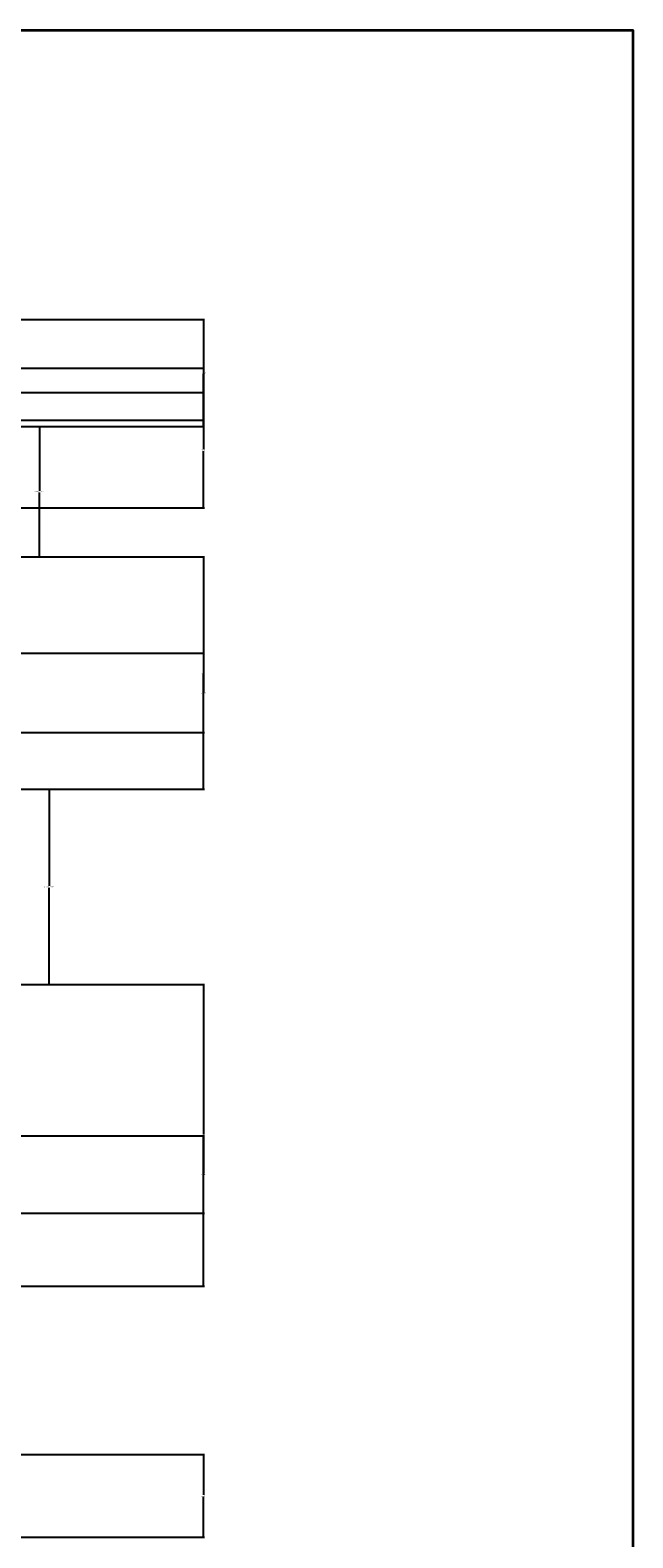
# Model space of a CAD drawing. Units: inches. Extents: x 2310 to 2937, y 1113 to 2410.
# Tile 23 of 23: x 2826 to 2937, y 2132 to 2410. Entities that reach past the tile are written whole.
import ezdxf

# ---------------------------------------------------------------- set-up
doc = ezdxf.new("R2010")
doc.units = ezdxf.units.IN
doc.layers.add('A-ANNO-DIMS', color=2, linetype='Continuous', lineweight=18)
doc.layers.add('A-ANNO-TTLB', color=7, linetype='Continuous', lineweight=35)
doc.styles.get("Standard").update_dxf_attribs({"font": 'arial.ttf'})
doc.dimstyles.get("Standard").update_dxf_attribs({"dimtxt": 0.18, "dimasz": 0.18, "dimexe": 0.18, "dimexo": 0.0625, "dimgap": 0.09, "dimtad": 0, "dimtih": 1, "dimtoh": 1, "dimdec": 4, "dimzin": 0, "dimdsep": 46, "dimtxsty": 'Standard', "dimcen": 0.09, "dimadec": 0, "dimazin": 0, "dimtfac": 1, "dimtdec": 4, "dimtofl": 0, "dimtmove": 0, "dimatfit": 3, "dimfxl": 1, "dimtolj": 1, "dimtzin": 0, "dimarcsym": 0})

# ---------------------------------------------------------------- blocks, each defined once
blk = doc.blocks.new('*D29')
at = {"layer": 'A-ANNO-DIMS', "color": 0, "lineweight": -2, "transparency": 16777216}
for p, q in [((2824.05, 2336.76), (2827.77, 2336.76)), ((2827.59, 2336.58), (2827.59, 2324.94)), ((2827.59, 2312.94), (2827.59, 2324.58)), ((2824.05, 2312.76), (2827.77, 2312.76))]:
    blk.add_line(p, q, dxfattribs=at)
at = {"layer": 'A-ANNO-DIMS', "color": 0, "transparency": 16777216}
for points in [[(2827.56, 2336.58), (2827.62, 2336.58), (2827.59, 2336.76)], [(2827.56, 2312.94), (2827.62, 2312.94), (2827.59, 2312.76)]]:
    blk.add_solid(points, dxfattribs=at)
at = {"layer": 'Defpoints', "color": 0, "transparency": 16777216}
for p in [(2823.99, 2336.76), (2827.59, 2336.76), (2823.99, 2312.76)]:
    blk.add_point(p, dxfattribs=at)
at = {"layer": 'A-ANNO-DIMS', "color": 0, "transparency": 16777216, "insert": (2827.59, 2324.76), "char_height": 0.18, "attachment_point": 5}
blk.add_mtext('\\A1;WINDOW 24 TYP.', dxfattribs=at)
blk = doc.blocks.new('*D31')
at = {"layer": 'A-ANNO-DIMS', "color": 0, "lineweight": -2, "transparency": 16777216}
for p, q in [((2824.05, 2269.9), (2829.57, 2269.9)), ((2829.39, 2269.72), (2829.39, 2252.08)), ((2829.39, 2234.08), (2829.39, 2251.71)), ((2824.05, 2233.9), (2829.57, 2233.9))]:
    blk.add_line(p, q, dxfattribs=at)
at = {"layer": 'A-ANNO-DIMS', "color": 0, "transparency": 16777216}
for points in [[(2829.36, 2269.72), (2829.42, 2269.72), (2829.39, 2269.9)], [(2829.36, 2234.08), (2829.42, 2234.08), (2829.39, 2233.9)]]:
    blk.add_solid(points, dxfattribs=at)
at = {"layer": 'Defpoints', "color": 0, "transparency": 16777216}
for p in [(2823.99, 2269.9), (2829.39, 2269.9), (2823.99, 2233.9)]:
    blk.add_point(p, dxfattribs=at)
at = {"layer": 'A-ANNO-DIMS', "color": 0, "transparency": 16777216, "insert": (2829.39, 2251.9), "char_height": 0.18, "attachment_point": 5}
blk.add_mtext('\\A1;WINDOW 36 TYP.', dxfattribs=at)
blk = doc.blocks.new('*D49')
at = {"layer": 'A-ANNO-DIMS', "color": 0, "lineweight": -2, "transparency": 16777216}
for p, q in [((2824.05, 2233.9), (2858.02, 2233.9)), ((2857.84, 2233.72), (2857.84, 2206.28)), ((2857.84, 2178.48), (2857.84, 2205.92)), ((2824.05, 2178.3), (2858.02, 2178.3))]:
    blk.add_line(p, q, dxfattribs=at)
at = {"layer": 'A-ANNO-DIMS', "color": 0, "transparency": 16777216}
for points in [[(2857.81, 2233.72), (2857.87, 2233.72), (2857.84, 2233.9)], [(2857.81, 2178.48), (2857.87, 2178.48), (2857.84, 2178.3)]]:
    blk.add_solid(points, dxfattribs=at)
at = {"layer": 'Defpoints', "color": 0, "transparency": 16777216}
for p in [(2823.99, 2233.9), (2857.84, 2233.9), (2823.99, 2178.3)]:
    blk.add_point(p, dxfattribs=at)
at = {"layer": 'A-ANNO-DIMS', "color": 0, "transparency": 16777216, "insert": (2857.84, 2206.1), "char_height": 0.18, "attachment_point": 5}
blk.add_mtext('\\A1;55.6', dxfattribs=at)
blk = doc.blocks.new('*D50')
at = {"layer": 'A-ANNO-DIMS', "color": 0, "lineweight": -2, "transparency": 16777216}
for p, q in [((2824.05, 2312.76), (2858.02, 2312.76)), ((2857.84, 2312.58), (2857.84, 2291.51)), ((2857.84, 2270.08), (2857.84, 2291.15)), ((2824.05, 2269.9), (2858.02, 2269.9))]:
    blk.add_line(p, q, dxfattribs=at)
at = {"layer": 'A-ANNO-DIMS', "color": 0, "transparency": 16777216}
for points in [[(2857.81, 2312.58), (2857.87, 2312.58), (2857.84, 2312.76)], [(2857.81, 2270.08), (2857.87, 2270.08), (2857.84, 2269.9)]]:
    blk.add_solid(points, dxfattribs=at)
at = {"layer": 'Defpoints', "color": 0, "transparency": 16777216}
for p in [(2823.99, 2312.76), (2857.84, 2312.76), (2823.99, 2269.9)]:
    blk.add_point(p, dxfattribs=at)
at = {"layer": 'A-ANNO-DIMS', "color": 0, "transparency": 16777216, "insert": (2857.84, 2291.33), "char_height": 0.18, "attachment_point": 5}
blk.add_mtext('\\A1;42.86', dxfattribs=at)
blk = doc.blocks.new('*D51')
at = {"layer": 'A-ANNO-DIMS', "color": 0, "lineweight": -2, "transparency": 16777216}
for p, q in [((2824.05, 2356.51), (2858.02, 2356.51)), ((2857.84, 2356.33), (2857.84, 2346.82)), ((2857.84, 2336.94), (2857.84, 2346.46)), ((2824.05, 2336.76), (2858.02, 2336.76))]:
    blk.add_line(p, q, dxfattribs=at)
at = {"layer": 'A-ANNO-DIMS', "color": 0, "transparency": 16777216}
for points in [[(2857.81, 2356.33), (2857.87, 2356.33), (2857.84, 2356.51)], [(2857.81, 2336.94), (2857.87, 2336.94), (2857.84, 2336.76)]]:
    blk.add_solid(points, dxfattribs=at)
at = {"layer": 'Defpoints', "color": 0, "transparency": 16777216}
for p in [(2823.99, 2356.51), (2857.84, 2356.51), (2823.99, 2336.76)]:
    blk.add_point(p, dxfattribs=at)
at = {"layer": 'A-ANNO-DIMS', "color": 0, "transparency": 16777216, "insert": (2857.84, 2346.64), "char_height": 0.18, "attachment_point": 5}
blk.add_mtext('\\A1;19.754', dxfattribs=at)
blk = doc.blocks.new('*D52')
at = {"layer": 'A-ANNO-DIMS', "color": 0, "lineweight": -2, "transparency": 16777216}
for p, q in [((2403.55, 2347.51), (2858.02, 2347.51)), ((2857.84, 2347.33), (2857.84, 2342.9)), ((2857.84, 2338.1), (2857.84, 2342.54)), ((2403.55, 2337.92), (2858.02, 2337.92))]:
    blk.add_line(p, q, dxfattribs=at)
at = {"layer": 'A-ANNO-DIMS', "color": 0, "transparency": 16777216}
for points in [[(2857.81, 2347.33), (2857.87, 2347.33), (2857.84, 2347.51)], [(2857.81, 2338.1), (2857.87, 2338.1), (2857.84, 2337.92)]]:
    blk.add_solid(points, dxfattribs=at)
at = {"layer": 'Defpoints', "color": 0, "transparency": 16777216}
for p in [(2403.49, 2347.51), (2403.49, 2337.92), (2857.84, 2337.92)]:
    blk.add_point(p, dxfattribs=at)
at = {"layer": 'A-ANNO-DIMS', "color": 0, "transparency": 16777216, "insert": (2857.84, 2342.72), "char_height": 0.18, "attachment_point": 5}
blk.add_mtext('\\A1;9.59', dxfattribs=at)
blk = doc.blocks.new('*D53')
at = {"layer": 'A-ANNO-DIMS', "color": 0, "lineweight": -2, "transparency": 16777216}
for p, q in [((2403.55, 2295.01), (2858.02, 2295.01)), ((2857.84, 2294.83), (2857.84, 2287.87)), ((2857.84, 2280.55), (2857.84, 2287.51)), ((2403.55, 2280.37), (2858.02, 2280.37))]:
    blk.add_line(p, q, dxfattribs=at)
at = {"layer": 'A-ANNO-DIMS', "color": 0, "transparency": 16777216}
for points in [[(2857.81, 2294.83), (2857.87, 2294.83), (2857.84, 2295.01)], [(2857.81, 2280.55), (2857.87, 2280.55), (2857.84, 2280.37)]]:
    blk.add_solid(points, dxfattribs=at)
at = {"layer": 'Defpoints', "color": 0, "transparency": 16777216}
for p in [(2403.49, 2295.01), (2403.49, 2280.37), (2857.84, 2280.37)]:
    blk.add_point(p, dxfattribs=at)
at = {"layer": 'A-ANNO-DIMS', "color": 0, "transparency": 16777216, "insert": (2857.84, 2287.69), "char_height": 0.18, "attachment_point": 5}
blk.add_mtext('\\A1;14.644', dxfattribs=at)
blk = doc.blocks.new('*D54')
at = {"layer": 'A-ANNO-DIMS', "color": 0, "lineweight": -2, "transparency": 16777216}
for p, q in [((2403.55, 2206.01), (2858.02, 2206.01)), ((2857.84, 2205.83), (2857.84, 2199.07)), ((2857.84, 2191.94), (2857.84, 2198.7)), ((2403.55, 2191.76), (2858.02, 2191.76))]:
    blk.add_line(p, q, dxfattribs=at)
at = {"layer": 'A-ANNO-DIMS', "color": 0, "transparency": 16777216}
for points in [[(2857.81, 2205.83), (2857.87, 2205.83), (2857.84, 2206.01)], [(2857.81, 2191.94), (2857.87, 2191.94), (2857.84, 2191.76)]]:
    blk.add_solid(points, dxfattribs=at)
at = {"layer": 'Defpoints', "color": 0, "transparency": 16777216}
for p in [(2403.49, 2206.01), (2403.49, 2191.76), (2857.84, 2191.76)]:
    blk.add_point(p, dxfattribs=at)
at = {"layer": 'A-ANNO-DIMS', "color": 0, "transparency": 16777216, "insert": (2857.84, 2198.89), "char_height": 0.18, "attachment_point": 5}
blk.add_mtext('\\A1;14.255', dxfattribs=at)
blk = doc.blocks.new('*D59')
at = {"layer": 'A-ANNO-DIMS', "color": 0, "lineweight": -2, "transparency": 16777216}
for p, q in [((2480.05, 2343.04), (2858.02, 2343.04)), ((2857.84, 2342.86), (2857.84, 2332.58)), ((2857.84, 2321.94), (2857.84, 2332.22)), ((2480.05, 2321.76), (2858.02, 2321.76))]:
    blk.add_line(p, q, dxfattribs=at)
at = {"layer": 'A-ANNO-DIMS', "color": 0, "transparency": 16777216}
for points in [[(2857.81, 2342.86), (2857.87, 2342.86), (2857.84, 2343.04)], [(2857.81, 2321.94), (2857.87, 2321.94), (2857.84, 2321.76)]]:
    blk.add_solid(points, dxfattribs=at)
at = {"layer": 'Defpoints', "color": 0, "transparency": 16777216}
for p in [(2479.99, 2343.04), (2857.84, 2343.04), (2479.99, 2321.76)]:
    blk.add_point(p, dxfattribs=at)
at = {"layer": 'A-ANNO-DIMS', "color": 0, "transparency": 16777216, "insert": (2857.84, 2332.4), "char_height": 0.18, "attachment_point": 5}
blk.add_mtext('\\A1;21.28', dxfattribs=at)
blk = doc.blocks.new('*D70')
at = {"layer": 'A-ANNO-DIMS', "color": 0, "lineweight": -2, "transparency": 16777216}
for p, q in [((2475.96, 2147.28), (2858.02, 2147.28)), ((2857.84, 2147.1), (2857.84, 2139.83)), ((2857.84, 2132.2), (2857.84, 2139.47)), ((2475.96, 2132.02), (2858.02, 2132.02))]:
    blk.add_line(p, q, dxfattribs=at)
at = {"layer": 'A-ANNO-DIMS', "color": 0, "transparency": 16777216}
for points in [[(2857.81, 2147.1), (2857.87, 2147.1), (2857.84, 2147.28)], [(2857.81, 2132.2), (2857.87, 2132.2), (2857.84, 2132.02)]]:
    blk.add_solid(points, dxfattribs=at)
at = {"layer": 'Defpoints', "color": 0, "transparency": 16777216}
for p in [(2475.89, 2147.28), (2857.84, 2147.28), (2475.89, 2132.02)]:
    blk.add_point(p, dxfattribs=at)
at = {"layer": 'A-ANNO-DIMS', "color": 0, "transparency": 16777216, "insert": (2857.84, 2139.65), "char_height": 0.18, "attachment_point": 5}
blk.add_mtext('\\A1;15.257', dxfattribs=at)

msp = doc.modelspace()

# ---------------------------------------------------------------- linework, layer by layer
at = {"layer": 'A-ANNO-TTLB'}
msp.add_lwpolyline([(2310.2498, 2409.8427), (2937.0534, 2409.8427), (2937.0534, 1616.036), (2310.2498, 1616.036)], close=True, dxfattribs=at)

# ---------------------------------------------------------------- dimensions: what is measured, and where the dimension line sits
at = {"layer": 'A-ANNO-DIMS'}
for base, p1, p2, override, picture, middle in [((2857.8359, 2356.5139), (2823.9859, 2336.76), (2823.9859, 2356.5139), {"dimdec": 3, "dimlfac": 1, "dimrnd": 0, "dimzin": 0, "dimdsep": 46, "dimlunit": 2}, '*D51', (2857.8359, 2346.637)), ((2857.8359, 2337.9231), (2403.4859, 2347.5139), (2403.4859, 2337.9231), {"dimdec": 2, "dimlfac": 1, "dimrnd": 0, "dimzin": 0, "dimdsep": 46, "dimlunit": 2}, '*D52', (2857.8359, 2342.7185)), ((2857.8359, 2343.0384), (2479.9859, 2321.7598), (2479.9859, 2343.0384), {"dimdec": 2, "dimlfac": 1, "dimrnd": 0, "dimzin": 0, "dimdsep": 46, "dimlunit": 2}, '*D59', (2857.8359, 2332.3991)), ((2857.8359, 2312.76), (2823.9859, 2269.8977), (2823.9859, 2312.76), {"dimdec": 2, "dimlfac": 1, "dimrnd": 0, "dimzin": 0, "dimdsep": 46, "dimlunit": 2}, '*D50', (2857.8359, 2291.3288)), ((2857.8359, 2280.3697), (2403.4859, 2295.0139), (2403.4859, 2280.3697), {"dimdec": 3, "dimlfac": 1, "dimrnd": 0, "dimzin": 0, "dimdsep": 46, "dimlunit": 2}, '*D53', (2857.8359, 2287.6918)), ((2857.8359, 2233.8977), (2823.9859, 2178.3027), (2823.9859, 2233.8977), {"dimdec": 1, "dimlfac": 1, "dimrnd": 0, "dimzin": 0, "dimdsep": 46, "dimlunit": 2}, '*D49', (2857.8359, 2206.1002)), ((2857.8359, 2191.7587), (2403.4859, 2206.0139), (2403.4859, 2191.7587), {"dimdec": 3, "dimlfac": 1, "dimrnd": 0, "dimzin": 0, "dimdsep": 46, "dimlunit": 2}, '*D54', (2857.8359, 2198.8863)), ((2857.8359, 2147.2815), (2475.8929, 2132.0241), (2475.8929, 2147.2815), {"dimdec": 3, "dimlfac": 1, "dimrnd": 0, "dimzin": 0, "dimdsep": 46, "dimlunit": 2}, '*D70', (2857.8359, 2139.6528))]:
    dim = msp.add_linear_dim(base=base, p1=p1, p2=p2, angle=90, dimstyle='Standard', override=override, dxfattribs=at)
    dim.commit()
    dim.dimension.update_dxf_attribs({"geometry": picture, "text_midpoint": middle})
for base, p1, p2, picture, middle in [((2827.5859, 2336.76), (2823.9859, 2312.76), (2823.9859, 2336.76), '*D29', (2827.5859, 2324.76)), ((2829.3859, 2269.8977), (2823.9859, 2233.8977), (2823.9859, 2269.8977), '*D31', (2829.3859, 2251.8977))]:
    dim = msp.add_linear_dim(base=base, p1=p1, p2=p2, angle=90, text='WINDOW <> TYP.', dimstyle='Standard', override={"dimdec": 0, "dimlfac": 1, "dimrnd": 0, "dimzin": 0, "dimdsep": 46, "dimlunit": 2}, dxfattribs=at)
    dim.commit()
    dim.dimension.update_dxf_attribs({"geometry": picture, "text_midpoint": middle})

doc.saveas('drawing.dxf')
